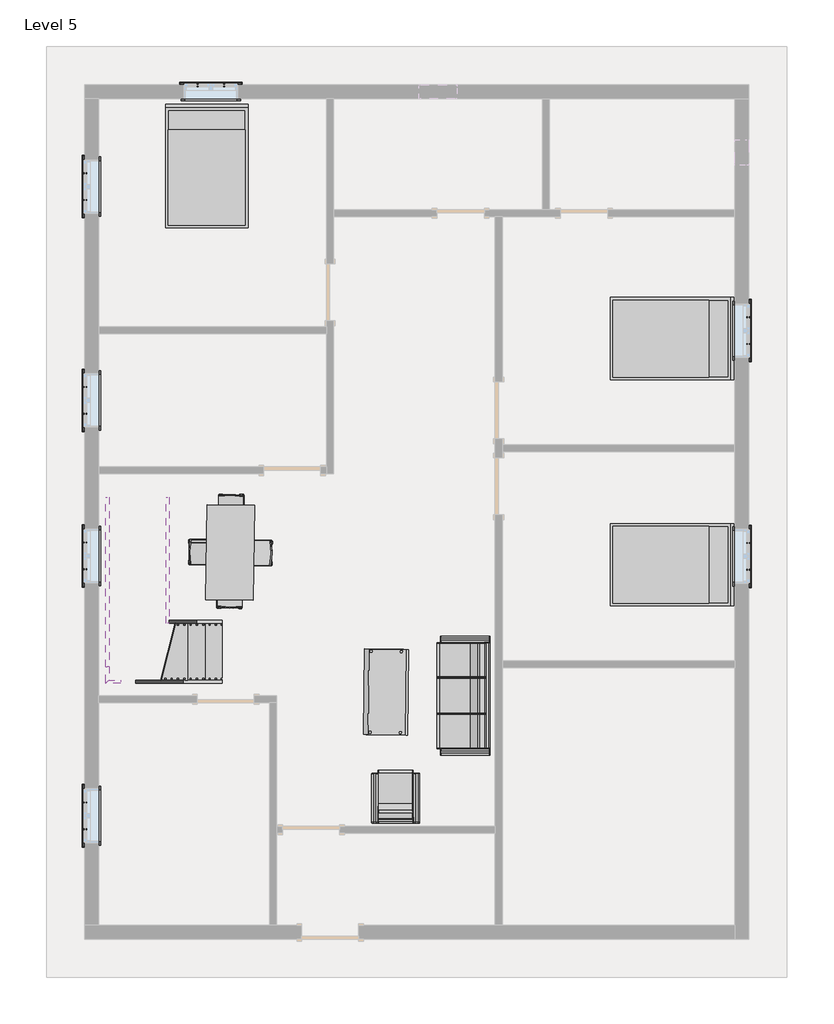
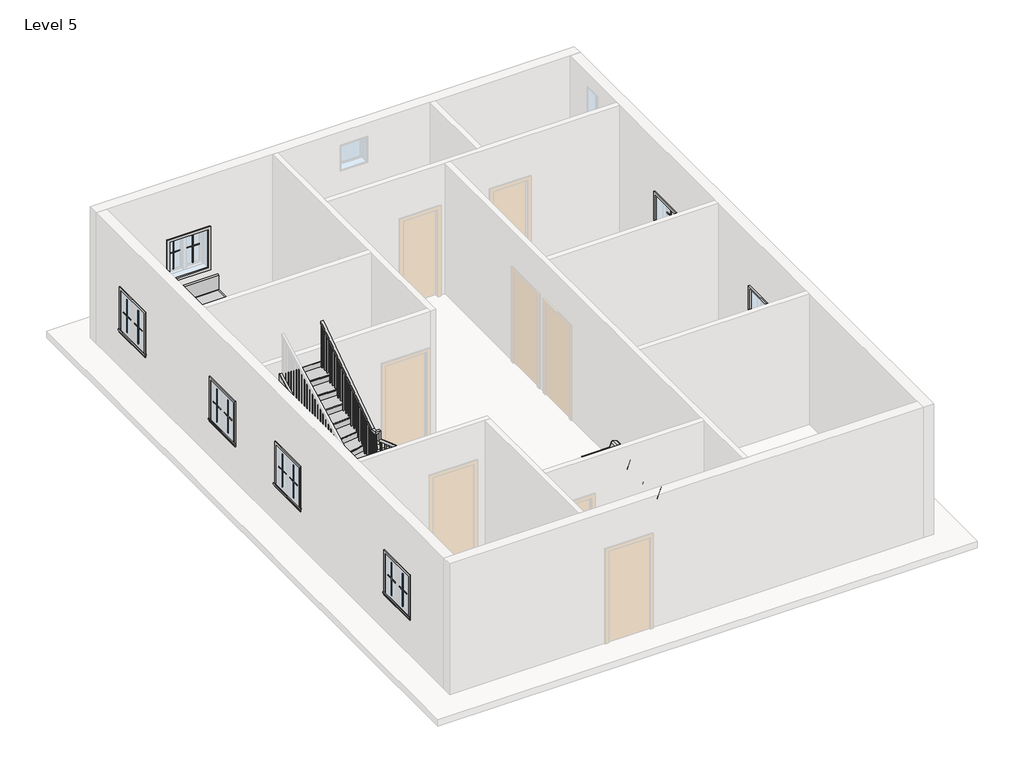
# One storey, part 2 of 2: 29 proxies, 6 furniture elements, 6 members, 1 railing, 1 stair flight.
"""IFC4 building model written with IfcOpenShell, lengths in millimetres."""

from ifc_helpers import new_model, si_unit, frame, origin, place, context, project, spatial, polyline, outline, extrude, faceted_brep, transform, mapped, element, save
from components import modern_coffee_table_17989_modern_coffee_table_17989_d3a860c8, muntin_pattern_2x2_muntin_pattern_2x2_b3fe6957, muntin_pattern_2x2_muntin_pattern_2x2_3e0ecaf2, trim_window_exterior_flat_with_sill_41619996, trim_window_interior_flat_picture_frame_51c85655, furniture_2fc85b74, furniture_29a9adb8, furniture_57072a26, furniture_f28dd14e, furniture_402a1f5e, bed_17739_bed_17739_15c61121, dining_table_w_chairs_11374_0cdfc61b, stair_flight_14253777

model = new_model("IFC4")

# Units and contexts
model_context = context("Model", 3, world=origin())
ifc_project = project(units=[si_unit("LENGTHUNIT", "METRE", prefix="MILLI")], contexts=[model_context])

# Site, building, storey
site = spatial("IfcSite", under=ifc_project)
building = spatial("IfcBuilding", under=site)
storey = spatial("IfcBuildingStorey", under=building, Name="Level 5", Elevation=9601.2)

# Proxies
placement = place(None, origin())
modern_coffee_table_17989_modern_coffee_table_17989_shape = modern_coffee_table_17989_modern_coffee_table_17989_d3a860c8(model_context)
element("IfcBuildingElementProxy", 1, Name="Modern_Coffee_Table_17989 : Modern_Coffee_Table_17989", ObjectType="Modern_Coffee_Table_17989 : Modern_Coffee_Table_17989", at=placement, inside=storey, context=model_context, shape_type="MappedRepresentation", body=[
    mapped(modern_coffee_table_17989_modern_coffee_table_17989_shape, transform((-2106.8718825, -2116.758017, 9601.2), x_axis=(0.012591066442684793, 0.9999207293810025, 0.0), y_axis=(-0.9999207293810025, 0.012591066442684793, 0.0), z_axis=(0.0, 0.0, 1.0))),
])
muntin_pattern_2x2_muntin_pattern_2x2_shape = muntin_pattern_2x2_muntin_pattern_2x2_b3fe6957(model_context)
element("IfcBuildingElementProxy", 2, Name="Muntin Pattern_2x2 : Muntin Pattern_2x2", ObjectType="Muntin Pattern_2x2 : Muntin Pattern_2x2", at=placement, inside=storey, context=model_context, shape_type="MappedRepresentation", body=[
    mapped(muntin_pattern_2x2_muntin_pattern_2x2_shape, transform((-4775.9474931, 7386.6685985, 10585.45), x_axis=(1.0, 0.0, 0.0), y_axis=(0.0, 1.0, 0.0), z_axis=(0.0, 0.0, 1.0))),
])
element("IfcBuildingElementProxy", 3, Name="Muntin Pattern_2x2 : Muntin Pattern_2x2", ObjectType="Muntin Pattern_2x2 : Muntin Pattern_2x2", at=placement, inside=storey, context=model_context, shape_type="MappedRepresentation", body=[
    mapped(muntin_pattern_2x2_muntin_pattern_2x2_shape, transform((4068.0150069, 3660.8060985, 10585.45), x_axis=(0.0, -1.0, 0.0), y_axis=(1.0, 0.0, 0.0), z_axis=(0.0, 0.0, 1.0))),
])
element("IfcBuildingElementProxy", 4, Name="Muntin Pattern_2x2 : Muntin Pattern_2x2", ObjectType="Muntin Pattern_2x2 : Muntin Pattern_2x2", at=placement, inside=storey, context=model_context, shape_type="MappedRepresentation", body=[
    mapped(muntin_pattern_2x2_muntin_pattern_2x2_shape, transform((4068.0150069, 40.9802908, 10585.45), x_axis=(0.0, -1.0, 0.0), y_axis=(1.0, 0.0, 0.0), z_axis=(0.0, 0.0, 1.0))),
])
element("IfcBuildingElementProxy", 5, Name="Muntin Pattern_2x2 : Muntin Pattern_2x2", ObjectType="Muntin Pattern_2x2 : Muntin Pattern_2x2", at=placement, inside=storey, context=model_context, shape_type="MappedRepresentation", body=[
    mapped(muntin_pattern_2x2_muntin_pattern_2x2_shape, transform((-6580.9349931, 2114.5810985, 10585.45), x_axis=(0.0, 1.0, 0.0), y_axis=(-1.0, 0.0, 0.0), z_axis=(0.0, 0.0, 1.0))),
])
element("IfcBuildingElementProxy", 6, Name="Muntin Pattern_2x2 : Muntin Pattern_2x2", ObjectType="Muntin Pattern_2x2 : Muntin Pattern_2x2", at=placement, inside=storey, context=model_context, shape_type="MappedRepresentation", body=[
    mapped(muntin_pattern_2x2_muntin_pattern_2x2_shape, transform((-6580.9349931, 5543.5810985, 10585.45), x_axis=(0.0, 1.0, 0.0), y_axis=(-1.0, 0.0, 0.0), z_axis=(0.0, 0.0, 1.0))),
])
element("IfcBuildingElementProxy", 7, Name="Muntin Pattern_2x2 : Muntin Pattern_2x2", ObjectType="Muntin Pattern_2x2 : Muntin Pattern_2x2", at=placement, inside=storey, context=model_context, shape_type="MappedRepresentation", body=[
    mapped(muntin_pattern_2x2_muntin_pattern_2x2_shape, transform((-6580.9349931, -4549.7439015, 10585.45), x_axis=(0.0, 1.0, 0.0), y_axis=(-1.0, 0.0, 0.0), z_axis=(0.0, 0.0, 1.0))),
])
element("IfcBuildingElementProxy", 8, Name="Muntin Pattern_2x2 : Muntin Pattern_2x2", ObjectType="Muntin Pattern_2x2 : Muntin Pattern_2x2", at=placement, inside=storey, context=model_context, shape_type="MappedRepresentation", body=[
    mapped(muntin_pattern_2x2_muntin_pattern_2x2_shape, transform((-6580.9349931, -380.9689015, 10585.45), x_axis=(0.0, 1.0, 0.0), y_axis=(-1.0, 0.0, 0.0), z_axis=(0.0, 0.0, 1.0))),
])
muntin_pattern_2x2_muntin_pattern_2x2_2_shape = muntin_pattern_2x2_muntin_pattern_2x2_3e0ecaf2(model_context)
element("IfcBuildingElementProxy", 9, Name="Muntin Pattern_2x2 : Muntin Pattern_2x2", ObjectType="Muntin Pattern_2x2 : Muntin Pattern_2x2", at=placement, inside=storey, context=model_context, shape_type="MappedRepresentation", body=[
    mapped(muntin_pattern_2x2_muntin_pattern_2x2_2_shape, transform((-4347.3224931, 7386.6685985, 10585.45), x_axis=(-1.0, 0.0, 0.0), y_axis=(0.0, -1.0, 0.0), z_axis=(0.0, 0.0, 1.0))),
])
element("IfcBuildingElementProxy", 10, Name="Muntin Pattern_2x2 : Muntin Pattern_2x2", ObjectType="Muntin Pattern_2x2 : Muntin Pattern_2x2", at=placement, inside=storey, context=model_context, shape_type="MappedRepresentation", body=[
    mapped(muntin_pattern_2x2_muntin_pattern_2x2_2_shape, transform((4068.0150069, 3232.1810985, 10585.45), x_axis=(0.0, 1.0, 0.0), y_axis=(-1.0, 0.0, 0.0), z_axis=(0.0, 0.0, 1.0))),
])
element("IfcBuildingElementProxy", 11, Name="Muntin Pattern_2x2 : Muntin Pattern_2x2", ObjectType="Muntin Pattern_2x2 : Muntin Pattern_2x2", at=placement, inside=storey, context=model_context, shape_type="MappedRepresentation", body=[
    mapped(muntin_pattern_2x2_muntin_pattern_2x2_2_shape, transform((4068.0150069, -387.6447092, 10585.45), x_axis=(0.0, 1.0, 0.0), y_axis=(-1.0, 0.0, 0.0), z_axis=(0.0, 0.0, 1.0))),
])
element("IfcBuildingElementProxy", 12, Name="Muntin Pattern_2x2 : Muntin Pattern_2x2", ObjectType="Muntin Pattern_2x2 : Muntin Pattern_2x2", at=placement, inside=storey, context=model_context, shape_type="MappedRepresentation", body=[
    mapped(muntin_pattern_2x2_muntin_pattern_2x2_2_shape, transform((-6580.9349931, 2543.2060985, 10585.45), x_axis=(0.0, -1.0, 0.0), y_axis=(1.0, 0.0, 0.0), z_axis=(0.0, 0.0, 1.0))),
])
element("IfcBuildingElementProxy", 13, Name="Muntin Pattern_2x2 : Muntin Pattern_2x2", ObjectType="Muntin Pattern_2x2 : Muntin Pattern_2x2", at=placement, inside=storey, context=model_context, shape_type="MappedRepresentation", body=[
    mapped(muntin_pattern_2x2_muntin_pattern_2x2_2_shape, transform((-6580.9349931, 5972.2060985, 10585.45), x_axis=(0.0, -1.0, 0.0), y_axis=(1.0, 0.0, 0.0), z_axis=(0.0, 0.0, 1.0))),
])
element("IfcBuildingElementProxy", 14, Name="Muntin Pattern_2x2 : Muntin Pattern_2x2", ObjectType="Muntin Pattern_2x2 : Muntin Pattern_2x2", at=placement, inside=storey, context=model_context, shape_type="MappedRepresentation", body=[
    mapped(muntin_pattern_2x2_muntin_pattern_2x2_2_shape, transform((-6580.9349931, -4121.1189015, 10585.45), x_axis=(0.0, -1.0, 0.0), y_axis=(1.0, 0.0, 0.0), z_axis=(0.0, 0.0, 1.0))),
])
element("IfcBuildingElementProxy", 15, Name="Muntin Pattern_2x2 : Muntin Pattern_2x2", ObjectType="Muntin Pattern_2x2 : Muntin Pattern_2x2", at=placement, inside=storey, context=model_context, shape_type="MappedRepresentation", body=[
    mapped(muntin_pattern_2x2_muntin_pattern_2x2_2_shape, transform((-6580.9349931, 47.6560985, 10585.45), x_axis=(0.0, -1.0, 0.0), y_axis=(1.0, 0.0, 0.0), z_axis=(0.0, 0.0, 1.0))),
])
trim_window_exterior_flat_with_sill_shape = trim_window_exterior_flat_with_sill_41619996(model_context)
element("IfcBuildingElementProxy", 16, Name="Trim-Window-Exterior-Flat : with Sill", ObjectType="Trim-Window-Exterior-Flat : with Sill", at=placement, inside=storey, context=model_context, shape_type="MappedRepresentation", body=[
    mapped(trim_window_exterior_flat_with_sill_shape, transform((-4561.6349931, 7396.1935985, 11430.0), x_axis=(-1.0, 0.0, 0.0), y_axis=(0.0, 0.0, 1.0), z_axis=(0.0, 1.0, 0.0))),
])
element("IfcBuildingElementProxy", 17, Name="Trim-Window-Exterior-Flat : with Sill", ObjectType="Trim-Window-Exterior-Flat : with Sill", at=placement, inside=storey, context=model_context, shape_type="MappedRepresentation", body=[
    mapped(trim_window_exterior_flat_with_sill_shape, transform((4077.5400069, 3446.4935985, 11430.0), x_axis=(0.0, 1.0, 0.0), y_axis=(0.0, 0.0, 1.0), z_axis=(1.0, 0.0, 0.0))),
])
element("IfcBuildingElementProxy", 18, Name="Trim-Window-Exterior-Flat : with Sill", ObjectType="Trim-Window-Exterior-Flat : with Sill", at=placement, inside=storey, context=model_context, shape_type="MappedRepresentation", body=[
    mapped(trim_window_exterior_flat_with_sill_shape, transform((4077.5400069, -173.3322092, 11430.0), x_axis=(0.0, 1.0, 0.0), y_axis=(0.0, 0.0, 1.0), z_axis=(1.0, 0.0, 0.0))),
])
element("IfcBuildingElementProxy", 19, Name="Trim-Window-Exterior-Flat : with Sill", ObjectType="Trim-Window-Exterior-Flat : with Sill", at=placement, inside=storey, context=model_context, shape_type="MappedRepresentation", body=[
    mapped(trim_window_exterior_flat_with_sill_shape, transform((-6590.4599931, 2328.8935985, 11430.0), x_axis=(0.0, -1.0, 0.0), y_axis=(0.0, 0.0, 1.0), z_axis=(-1.0, 0.0, 0.0))),
])
element("IfcBuildingElementProxy", 20, Name="Trim-Window-Exterior-Flat : with Sill", ObjectType="Trim-Window-Exterior-Flat : with Sill", at=placement, inside=storey, context=model_context, shape_type="MappedRepresentation", body=[
    mapped(trim_window_exterior_flat_with_sill_shape, transform((-6590.4599931, 5757.8935985, 11430.0), x_axis=(0.0, -1.0, 0.0), y_axis=(0.0, 0.0, 1.0), z_axis=(-1.0, 0.0, 0.0))),
])
element("IfcBuildingElementProxy", 21, Name="Trim-Window-Exterior-Flat : with Sill", ObjectType="Trim-Window-Exterior-Flat : with Sill", at=placement, inside=storey, context=model_context, shape_type="MappedRepresentation", body=[
    mapped(trim_window_exterior_flat_with_sill_shape, transform((-6590.4599931, -4335.4314015, 11430.0), x_axis=(0.0, -1.0, 0.0), y_axis=(0.0, 0.0, 1.0), z_axis=(-1.0, 0.0, 0.0))),
])
element("IfcBuildingElementProxy", 22, Name="Trim-Window-Exterior-Flat : with Sill", ObjectType="Trim-Window-Exterior-Flat : with Sill", at=placement, inside=storey, context=model_context, shape_type="MappedRepresentation", body=[
    mapped(trim_window_exterior_flat_with_sill_shape, transform((-6590.4599931, -166.6564015, 11430.0), x_axis=(0.0, -1.0, 0.0), y_axis=(0.0, 0.0, 1.0), z_axis=(-1.0, 0.0, 0.0))),
])
trim_window_interior_flat_picture_frame_shape = trim_window_interior_flat_picture_frame_51c85655(model_context)
element("IfcBuildingElementProxy", 23, Name="Trim-Window-Interior-Flat : Picture Frame", ObjectType="Trim-Window-Interior-Flat : Picture Frame", at=placement, inside=storey, context=model_context, shape_type="MappedRepresentation", body=[
    mapped(trim_window_interior_flat_picture_frame_shape, transform((-4561.6349931, 7167.5935985, 11430.0), x_axis=(1.0, 0.0, 0.0), y_axis=(0.0, 0.0, 1.0), z_axis=(0.0, -1.0, 0.0))),
])
element("IfcBuildingElementProxy", 24, Name="Trim-Window-Interior-Flat : Picture Frame", ObjectType="Trim-Window-Interior-Flat : Picture Frame", at=placement, inside=storey, context=model_context, shape_type="MappedRepresentation", body=[
    mapped(trim_window_interior_flat_picture_frame_shape, transform((3848.9400069, 3446.4935985, 11430.0), x_axis=(0.0, -1.0, 0.0), y_axis=(0.0, 0.0, 1.0), z_axis=(-1.0, 0.0, 0.0))),
])
element("IfcBuildingElementProxy", 25, Name="Trim-Window-Interior-Flat : Picture Frame", ObjectType="Trim-Window-Interior-Flat : Picture Frame", at=placement, inside=storey, context=model_context, shape_type="MappedRepresentation", body=[
    mapped(trim_window_interior_flat_picture_frame_shape, transform((3848.9400069, -173.3322092, 11430.0), x_axis=(0.0, -1.0, 0.0), y_axis=(0.0, 0.0, 1.0), z_axis=(-1.0, 0.0, 0.0))),
])
element("IfcBuildingElementProxy", 26, Name="Trim-Window-Interior-Flat : Picture Frame", ObjectType="Trim-Window-Interior-Flat : Picture Frame", at=placement, inside=storey, context=model_context, shape_type="MappedRepresentation", body=[
    mapped(trim_window_interior_flat_picture_frame_shape, transform((-6361.8599931, 2328.8935985, 11430.0), x_axis=(0.0, 1.0, 0.0), y_axis=(0.0, 0.0, 1.0), z_axis=(1.0, 0.0, 0.0))),
])
element("IfcBuildingElementProxy", 27, Name="Trim-Window-Interior-Flat : Picture Frame", ObjectType="Trim-Window-Interior-Flat : Picture Frame", at=placement, inside=storey, context=model_context, shape_type="MappedRepresentation", body=[
    mapped(trim_window_interior_flat_picture_frame_shape, transform((-6361.8599931, 5757.8935985, 11430.0), x_axis=(0.0, 1.0, 0.0), y_axis=(0.0, 0.0, 1.0), z_axis=(1.0, 0.0, 0.0))),
])
element("IfcBuildingElementProxy", 28, Name="Trim-Window-Interior-Flat : Picture Frame", ObjectType="Trim-Window-Interior-Flat : Picture Frame", at=placement, inside=storey, context=model_context, shape_type="MappedRepresentation", body=[
    mapped(trim_window_interior_flat_picture_frame_shape, transform((-6361.8599931, -4335.4314015, 11430.0), x_axis=(0.0, 1.0, 0.0), y_axis=(0.0, 0.0, 1.0), z_axis=(1.0, 0.0, 0.0))),
])
element("IfcBuildingElementProxy", 29, Name="Trim-Window-Interior-Flat : Picture Frame", ObjectType="Trim-Window-Interior-Flat : Picture Frame", at=placement, inside=storey, context=model_context, shape_type="MappedRepresentation", body=[
    mapped(trim_window_interior_flat_picture_frame_shape, transform((-6361.8599931, -166.6564015, 11430.0), x_axis=(0.0, 1.0, 0.0), y_axis=(0.0, 0.0, 1.0), z_axis=(1.0, 0.0, 0.0))),
])

# Furniture
furniture_shape = furniture_2fc85b74(model_context)
furniture_2_shape = furniture_29a9adb8(model_context)
furniture_3_shape = furniture_57072a26(model_context)
element("IfcFurniture", 30, at=placement, inside=storey, context=model_context, shape_type="MappedRepresentation", body=[
    mapped(furniture_shape, transform((-877.7263413, -2408.2064015, 9601.2), x_axis=(0.0, -1.0, 0.0), y_axis=(1.0, 0.0, 0.0), z_axis=(0.0, 0.0, 1.0))),
    mapped(furniture_2_shape, transform((-877.7263413, -2408.2064015, 9601.2), x_axis=(0.0, -1.0, 0.0), y_axis=(1.0, 0.0, 0.0), z_axis=(0.0, 0.0, 1.0))),
    mapped(furniture_3_shape, transform((-877.7263413, -2408.2064015, 9601.2), x_axis=(0.0, -1.0, 0.0), y_axis=(1.0, 0.0, 0.0), z_axis=(0.0, 0.0, 1.0))),
])
furniture_4_shape = furniture_f28dd14e(model_context)
furniture_5_shape = furniture_402a1f5e(model_context)
element("IfcFurniture", 31, at=placement, inside=storey, context=model_context, shape_type="MappedRepresentation", body=[
    mapped(furniture_4_shape, transform((-1595.4975416, -3653.2527501, 9601.2), x_axis=(-1.0, 0.0, 0.0), y_axis=(0.0, -1.0, 0.0), z_axis=(0.0, 0.0, 1.0))),
    mapped(furniture_5_shape, transform((-1595.4975416, -3653.2527501, 9601.2), x_axis=(-1.0, 0.0, 0.0), y_axis=(0.0, -1.0, 0.0), z_axis=(0.0, 0.0, 1.0))),
])
bed_17739_bed_17739_shape = bed_17739_bed_17739_15c61121(model_context)
element("IfcFurniture", 32, ObjectType="Bed_17739 : Bed_17739", at=placement, inside=storey, context=model_context, shape_type="MappedRepresentation", body=[
    mapped(bed_17739_bed_17739_shape, transform((-4628.3099931, 6062.6935985, 9601.2), x_axis=(1.0, 0.0, 0.0), y_axis=(0.0, 1.0, 0.0), z_axis=(0.0, 0.0, 1.0))),
])
element("IfcFurniture", 33, ObjectType="Bed_17739 : Bed_17739", at=placement, inside=storey, context=model_context, shape_type="MappedRepresentation", body=[
    mapped(bed_17739_bed_17739_shape, transform((2820.2400069, 3319.4935985, 9601.2), x_axis=(0.0, -1.0, 0.0), y_axis=(1.0, 0.0, 0.0), z_axis=(0.0, 0.0, 1.0))),
])
element("IfcFurniture", 34, ObjectType="Bed_17739 : Bed_17739", at=placement, inside=storey, context=model_context, shape_type="MappedRepresentation", body=[
    mapped(bed_17739_bed_17739_shape, transform((2820.2400069, -307.008017, 9601.2), x_axis=(0.0, -1.0, 0.0), y_axis=(1.0, 0.0, 0.0), z_axis=(0.0, 0.0, 1.0))),
])
dining_table_w_chairs_11374_shape = dining_table_w_chairs_11374_0cdfc61b(model_context)
element("IfcFurniture", 35, ObjectType="Dining_Table_w_Chairs_11374", at=placement, inside=storey, context=model_context, shape_type="MappedRepresentation", body=[
    mapped(dining_table_w_chairs_11374_shape, transform((-4154.6586335, -131.9172641, 9601.2), x_axis=(0.015873758475140665, 0.9998740039584353, 0.0), y_axis=(-0.9998740039584353, 0.015873758475140665, 0.0), z_axis=(0.0, 0.0, 1.0))),
])

# Members
element("IfcMember", 36, ObjectType="Stringer - 2\" Width", at=placement, inside=storey, context=model_context, shape_type="SweptSolid", body=[
    extrude(outline(polyline([(10191.2562463, -4378.4230036), (10524.0849999, -4378.4230036), (11239.2971411, -6009.0851964), (10906.4683876, -6009.0851964), (10191.2562463, -4378.4230036)])), frame((0.0, -2211.3564015, 0.0), z_axis=(0.0, 1.0, 0.0), x_axis=(0.0, 0.0, 1.0)), (0.0, 0.0, 1.0), 50.8),
])
element("IfcMember", 37, ObjectType="Stringer - 2\" Width", at=placement, inside=storey, context=model_context, shape_type="SweptSolid", body=[
    extrude(outline(polyline([(-6009.0851964, -2160.5564015), (-6009.0851964, -2211.3564015), (-6247.5599931, -2211.3564015), (-6196.7599931, -2160.5564015), (-6009.0851964, -2160.5564015)])), frame((0.0, 0.0, 10906.4683876), z_axis=(0.0, 0.0, 1.0), x_axis=(1.0, 0.0, 0.0)), (0.0, 0.0, 1.0), 332.8287535),
])
element("IfcMember", 38, ObjectType="Stringer - 2\" Width", at=placement, inside=storey, context=model_context, shape_type="SweptSolid", body=[
    extrude(outline(polyline([(-6196.7599931, -2160.5564015), (-6247.5599931, -2211.3564015), (-6247.5599931, -1942.4030584), (-6196.7599931, -1942.4030584), (-6196.7599931, -2160.5564015)])), frame((0.0, 0.0, 10906.4683876), z_axis=(0.0, 0.0, 1.0), x_axis=(1.0, 0.0, 0.0)), (0.0, 0.0, 1.0), 332.8287535),
])
element("IfcMember", 39, ObjectType="Stringer - 2\" Width", at=placement, inside=storey, context=model_context, shape_type="SweptSolid", body=[
    extrude(outline(polyline([(-1942.4030584, 10906.4683876), (-1942.4030584, 11239.2971411), (775.380588, 12654.8189504), (775.380588, 12321.9901969), (-1942.4030584, 10906.4683876)])), frame((-6247.5599931, 0.0, 0.0), z_axis=(1.0, 0.0, 0.0), x_axis=(0.0, 1.0, 0.0)), (0.0, 0.0, 1.0), 50.8),
])
element("IfcMember", 40, ObjectType="Stringer - 2\" Width", at=placement, inside=storey, context=model_context, shape_type="SweptSolid", body=[
    extrude(outline(polyline([(10036.6922729, -4378.4230036), (10443.834734, -4378.4230036), (11199.3690344, -5231.5599931), (10792.2265733, -5231.5599931), (10036.6922729, -4378.4230036)])), frame((0.0, -1246.1564015, 0.0), z_axis=(0.0, 1.0, 0.0), x_axis=(0.0, 0.0, 1.0)), (0.0, 0.0, 1.0), 50.8),
])
element("IfcMember", 41, ObjectType="Stringer - 2\" Width", at=placement, inside=storey, context=model_context, shape_type="SweptSolid", body=[
    extrude(outline(polyline([(-1246.1564015, 10938.9212805), (-1246.1564015, 11311.1296678), (775.380588, 12727.9693854), (775.380588, 12355.7609981), (-1246.1564015, 10938.9212805)])), frame((-5282.3599931, 0.0, 0.0), z_axis=(1.0, 0.0, 0.0), x_axis=(0.0, 1.0, 0.0)), (0.0, 0.0, 1.0), 50.8),
])

# Railing
element("IfcRailing", 42, ObjectType="Handrail - Rectangular", at=placement, inside=storey, context=model_context, shape_type="SolidModel", body=[
    faceted_brep([(-4378.4230036, -1296.9564015, 11362.2666667), (-4378.4230036, -1296.9564015, 11297.3997378), (-4378.4230036, -1246.1564015, 11297.3997378), (-4378.4230036, -1246.1564015, 11362.2666667), (-5206.1599931, -1296.9564015, 12019.5201542), (-5256.9599931, -1296.9564015, 11994.990286), (-5256.9599931, -1246.1564015, 11994.990286), (-5206.1599931, -1246.1564015, 12019.5201542), (-5206.1599931, -1296.9564015, 12226.3172738), (-5256.9599931, -1296.9564015, 12175.5172738), (-5256.9599931, -1246.1564015, 12175.5172738), (-5206.1599931, -1246.1564015, 12226.3172738), (-5333.1599931, -1296.9564015, 12226.3172738), (-5333.1599931, -1296.9564015, 12175.5172738), (-5282.3599931, -1246.1564015, 12175.5172738), (-5282.3599931, -1246.1564015, 12226.3172738), (-5333.1599931, -1169.9564015, 12226.3172738), (-5333.1599931, -1154.1797661, 12175.5172738), (-5282.3599931, -1154.1797661, 12175.5172738), (-5282.3599931, -1169.9564015, 12226.3172738), (-5333.1599931, 775.380588, 13563.6), (-5282.3599931, 775.380588, 13563.6), (-5282.3599931, 775.380588, 13501.9546698), (-5333.1599931, 775.380588, 13501.9546698)], [[[0, 1, 2, 3]], [[1, 0, 4, 5]], [[2, 1, 5, 6]], [[3, 2, 6, 7]], [[0, 3, 7, 4]], [[5, 4, 8, 9]], [[6, 5, 9, 10]], [[7, 6, 10, 11]], [[4, 7, 11, 8]], [[9, 8, 12, 13]], [[10, 9, 13, 14]], [[11, 10, 14, 15]], [[8, 11, 15, 12]], [[13, 12, 16, 17]], [[14, 13, 17, 18]], [[15, 14, 18, 19]], [[12, 15, 19, 16]], [[20, 21, 22, 23]], [[17, 16, 20, 23]], [[18, 17, 23, 22]], [[19, 18, 22, 21]], [[16, 19, 21, 20]]]),
    extrude(outline(polyline([(750.9185985, 13485.1387679), (769.9685985, 13498.2343066), (769.9685985, 12479.8666667), (750.9185985, 12479.8666667), (750.9185985, 13485.1387679)])), frame((-5317.2849931, 0.0, 0.0), z_axis=(1.0, 0.0, 0.0), x_axis=(0.0, 1.0, 0.0)), (0.0, 0.0, 1.0), 19.05),
    extrude(outline(polyline([(649.3185985, 13415.2958945), (668.3685985, 13428.3914333), (668.3685985, 12479.8666667), (649.3185985, 12479.8666667), (649.3185985, 13415.2958945)])), frame((-5317.2849931, 0.0, 0.0), z_axis=(1.0, 0.0, 0.0), x_axis=(0.0, 1.0, 0.0)), (0.0, 0.0, 1.0), 19.05),
    extrude(outline(polyline([(547.7185985, 13345.4530212), (566.7685985, 13358.5485599), (566.7685985, 12479.8666667), (547.7185985, 12479.8666667), (547.7185985, 13345.4530212)])), frame((-5317.2849931, 0.0, 0.0), z_axis=(1.0, 0.0, 0.0), x_axis=(0.0, 1.0, 0.0)), (0.0, 0.0, 1.0), 19.05),
    extrude(outline(polyline([(446.1185985, 13275.6101478), (465.1685985, 13288.7056866), (465.1685985, 12310.5333333), (446.1185985, 12310.5333333), (446.1185985, 13275.6101478)])), frame((-5317.2849931, 0.0, 0.0), z_axis=(1.0, 0.0, 0.0), x_axis=(0.0, 1.0, 0.0)), (0.0, 0.0, 1.0), 19.05),
    extrude(outline(polyline([(344.5185985, 13205.7672745), (363.5685985, 13218.8628132), (363.5685985, 12310.5333333), (344.5185985, 12310.5333333), (344.5185985, 13205.7672745)])), frame((-5317.2849931, 0.0, 0.0), z_axis=(1.0, 0.0, 0.0), x_axis=(0.0, 1.0, 0.0)), (0.0, 0.0, 1.0), 19.05),
    extrude(outline(polyline([(242.9185985, 13135.9244011), (261.9685985, 13149.0199399), (261.9685985, 12310.5333333), (242.9185985, 12310.5333333), (242.9185985, 13135.9244011)])), frame((-5317.2849931, 0.0, 0.0), z_axis=(1.0, 0.0, 0.0), x_axis=(0.0, 1.0, 0.0)), (0.0, 0.0, 1.0), 19.05),
    extrude(outline(polyline([(141.3185985, 13066.0815278), (160.3685985, 13079.1770665), (160.3685985, 12141.2), (141.3185985, 12141.2), (141.3185985, 13066.0815278)])), frame((-5317.2849931, 0.0, 0.0), z_axis=(1.0, 0.0, 0.0), x_axis=(0.0, 1.0, 0.0)), (0.0, 0.0, 1.0), 19.05),
    extrude(outline(polyline([(39.7185985, 12996.2386544), (58.7685985, 13009.3341932), (58.7685985, 12141.2), (39.7185985, 12141.2), (39.7185985, 12996.2386544)])), frame((-5317.2849931, 0.0, 0.0), z_axis=(1.0, 0.0, 0.0), x_axis=(0.0, 1.0, 0.0)), (0.0, 0.0, 1.0), 19.05),
    extrude(outline(polyline([(-61.8814015, 12926.3957811), (-42.8314015, 12939.4913198), (-42.8314015, 11971.8666667), (-61.8814015, 11971.8666667), (-61.8814015, 12926.3957811)])), frame((-5317.2849931, 0.0, 0.0), z_axis=(1.0, 0.0, 0.0), x_axis=(0.0, 1.0, 0.0)), (0.0, 0.0, 1.0), 19.05),
    extrude(outline(polyline([(-163.4814015, 12856.5529077), (-144.4314015, 12869.6484465), (-144.4314015, 11971.8666667), (-163.4814015, 11971.8666667), (-163.4814015, 12856.5529077)])), frame((-5317.2849931, 0.0, 0.0), z_axis=(1.0, 0.0, 0.0), x_axis=(0.0, 1.0, 0.0)), (0.0, 0.0, 1.0), 19.05),
    extrude(outline(polyline([(-265.0814015, 12786.7100344), (-246.0314015, 12799.8055731), (-246.0314015, 11971.8666667), (-265.0814015, 11971.8666667), (-265.0814015, 12786.7100344)])), frame((-5317.2849931, 0.0, 0.0), z_axis=(1.0, 0.0, 0.0), x_axis=(0.0, 1.0, 0.0)), (0.0, 0.0, 1.0), 19.05),
    extrude(outline(polyline([(-366.6814015, 12716.867161), (-347.6314015, 12729.9626998), (-347.6314015, 11802.5333333), (-366.6814015, 11802.5333333), (-366.6814015, 12716.867161)])), frame((-5317.2849931, 0.0, 0.0), z_axis=(1.0, 0.0, 0.0), x_axis=(0.0, 1.0, 0.0)), (0.0, 0.0, 1.0), 19.05),
    extrude(outline(polyline([(-468.2814015, 12647.0242877), (-449.2314015, 12660.1198264), (-449.2314015, 11802.5333333), (-468.2814015, 11802.5333333), (-468.2814015, 12647.0242877)])), frame((-5317.2849931, 0.0, 0.0), z_axis=(1.0, 0.0, 0.0), x_axis=(0.0, 1.0, 0.0)), (0.0, 0.0, 1.0), 19.05),
    extrude(outline(polyline([(-569.8814015, 12577.1814143), (-550.8314015, 12590.2769531), (-550.8314015, 11802.5333333), (-569.8814015, 11802.5333333), (-569.8814015, 12577.1814143)])), frame((-5317.2849931, 0.0, 0.0), z_axis=(1.0, 0.0, 0.0), x_axis=(0.0, 1.0, 0.0)), (0.0, 0.0, 1.0), 19.05),
    extrude(outline(polyline([(-671.4814015, 12507.338541), (-652.4314015, 12520.4340797), (-652.4314015, 11633.2), (-671.4814015, 11633.2), (-671.4814015, 12507.338541)])), frame((-5317.2849931, 0.0, 0.0), z_axis=(1.0, 0.0, 0.0), x_axis=(0.0, 1.0, 0.0)), (0.0, 0.0, 1.0), 19.05),
    extrude(outline(polyline([(-773.0814015, 12437.4956676), (-754.0314015, 12450.5912064), (-754.0314015, 11633.2), (-773.0814015, 11633.2), (-773.0814015, 12437.4956676)])), frame((-5317.2849931, 0.0, 0.0), z_axis=(1.0, 0.0, 0.0), x_axis=(0.0, 1.0, 0.0)), (0.0, 0.0, 1.0), 19.05),
    extrude(outline(polyline([(-874.6814015, 12367.6527943), (-855.6314015, 12380.748333), (-855.6314015, 11463.8666667), (-874.6814015, 11463.8666667), (-874.6814015, 12367.6527943)])), frame((-5317.2849931, 0.0, 0.0), z_axis=(1.0, 0.0, 0.0), x_axis=(0.0, 1.0, 0.0)), (0.0, 0.0, 1.0), 19.05),
    extrude(outline(polyline([(-976.2814015, 12297.8099209), (-957.2314015, 12310.9054597), (-957.2314015, 11463.8666667), (-976.2814015, 11463.8666667), (-976.2814015, 12297.8099209)])), frame((-5317.2849931, 0.0, 0.0), z_axis=(1.0, 0.0, 0.0), x_axis=(0.0, 1.0, 0.0)), (0.0, 0.0, 1.0), 19.05),
    extrude(outline(polyline([(-1077.8814015, 12227.9670476), (-1058.8314015, 12241.0625863), (-1058.8314015, 11294.5333333), (-1077.8814015, 11294.5333333), (-1077.8814015, 12227.9670476)])), frame((-5317.2849931, 0.0, 0.0), z_axis=(1.0, 0.0, 0.0), x_axis=(0.0, 1.0, 0.0)), (0.0, 0.0, 1.0), 19.05),
    extrude(outline(polyline([(-1179.4814015, 12158.1241742), (-1160.4314015, 12171.219713), (-1160.4314015, 11294.5333333), (-1179.4814015, 11294.5333333), (-1179.4814015, 12158.1241742)])), frame((-5317.2849931, 0.0, 0.0), z_axis=(1.0, 0.0, 0.0), x_axis=(0.0, 1.0, 0.0)), (0.0, 0.0, 1.0), 19.05),
    extrude(outline(polyline([(-5283.2980036, -1262.0314015), (-5283.2980036, -1281.0814015), (-5302.3480036, -1281.0814015), (-5302.3480036, -1262.0314015), (-5283.2980036, -1262.0314015)])), frame((0.0, 0.0, 11125.2), z_axis=(0.0, 0.0, 1.0), x_axis=(1.0, 0.0, 0.0)), (0.0, 0.0, 1.0), 1050.3172738),
    extrude(outline(polyline([(11935.2295097, -5181.6980036), (11950.3559074, -5200.7480036), (10955.8666667, -5200.7480036), (10955.8666667, -5181.6980036), (11935.2295097, -5181.6980036)])), frame((0.0, -1281.0814015, 0.0), z_axis=(0.0, 1.0, 0.0), x_axis=(0.0, 0.0, 1.0)), (0.0, 0.0, 1.0), 19.05),
    extrude(outline(polyline([(11854.5553883, -5080.0980036), (11869.6817861, -5099.1480036), (10786.5333333, -5099.1480036), (10786.5333333, -5080.0980036), (11854.5553883, -5080.0980036)])), frame((0.0, -1281.0814015, 0.0), z_axis=(0.0, 1.0, 0.0), x_axis=(0.0, 0.0, 1.0)), (0.0, 0.0, 1.0), 19.05),
    extrude(outline(polyline([(11773.881267, -4978.4980036), (11789.0076647, -4997.5480036), (10786.5333333, -4997.5480036), (10786.5333333, -4978.4980036), (11773.881267, -4978.4980036)])), frame((0.0, -1281.0814015, 0.0), z_axis=(0.0, 1.0, 0.0), x_axis=(0.0, 0.0, 1.0)), (0.0, 0.0, 1.0), 19.05),
    extrude(outline(polyline([(11693.2071456, -4876.8980036), (11708.3335434, -4895.9480036), (10617.2, -4895.9480036), (10617.2, -4876.8980036), (11693.2071456, -4876.8980036)])), frame((0.0, -1281.0814015, 0.0), z_axis=(0.0, 1.0, 0.0), x_axis=(0.0, 0.0, 1.0)), (0.0, 0.0, 1.0), 19.05),
    extrude(outline(polyline([(11612.5330243, -4775.2980036), (11627.659422, -4794.3480036), (10617.2, -4794.3480036), (10617.2, -4775.2980036), (11612.5330243, -4775.2980036)])), frame((0.0, -1281.0814015, 0.0), z_axis=(0.0, 1.0, 0.0), x_axis=(0.0, 0.0, 1.0)), (0.0, 0.0, 1.0), 19.05),
    extrude(outline(polyline([(11531.8589029, -4673.6980036), (11546.9853007, -4692.7480036), (10617.2, -4692.7480036), (10617.2, -4673.6980036), (11531.8589029, -4673.6980036)])), frame((0.0, -1281.0814015, 0.0), z_axis=(0.0, 1.0, 0.0), x_axis=(0.0, 0.0, 1.0)), (0.0, 0.0, 1.0), 19.05),
    extrude(outline(polyline([(11451.1847816, -4572.0980036), (11466.3111793, -4591.1480036), (10447.8666667, -4591.1480036), (10447.8666667, -4572.0980036), (11451.1847816, -4572.0980036)])), frame((0.0, -1281.0814015, 0.0), z_axis=(0.0, 1.0, 0.0), x_axis=(0.0, 0.0, 1.0)), (0.0, 0.0, 1.0), 19.05),
    extrude(outline(polyline([(11370.5106602, -4470.4980036), (11385.637058, -4489.5480036), (10447.8666667, -4489.5480036), (10447.8666667, -4470.4980036), (11370.5106602, -4470.4980036)])), frame((0.0, -1281.0814015, 0.0), z_axis=(0.0, 1.0, 0.0), x_axis=(0.0, 0.0, 1.0)), (0.0, 0.0, 1.0), 19.05),
    extrude(outline(polyline([(-5298.2349931, -1262.0314015), (-5298.2349931, -1281.0814015), (-5317.2849931, -1281.0814015), (-5317.2849931, -1262.0314015), (-5298.2349931, -1262.0314015)])), frame((0.0, 0.0, 11125.2), z_axis=(0.0, 0.0, 1.0), x_axis=(1.0, 0.0, 0.0)), (0.0, 0.0, 1.0), 1050.3172738),
    extrude(outline(polyline([(756.330588, 13488.859131), (775.380588, 13501.9546698), (775.380588, 12479.8666667), (756.330588, 12479.8666667), (756.330588, 13488.859131)])), frame((-5317.2849931, 0.0, 0.0), z_axis=(1.0, 0.0, 0.0), x_axis=(0.0, 1.0, 0.0)), (0.0, 0.0, 1.0), 19.05),
    extrude(outline(polyline([(11297.3997378, -4378.4230036), (11312.5261355, -4397.4730036), (10447.8666667, -4397.4730036), (10447.8666667, -4378.4230036), (11297.3997378, -4378.4230036)])), frame((0.0, -1281.0814015, 0.0), z_axis=(0.0, 1.0, 0.0), x_axis=(0.0, 0.0, 1.0)), (0.0, 0.0, 1.0), 19.05),
])

# Stair flight
stair_flight_shape = stair_flight_14253777(model_context)
element("IfcStairFlight", 43, ObjectType="2\" Tread 1\" Nosing 1/4\" Riser", at=placement, inside=storey, context=model_context, shape_type="MappedRepresentation", body=[
    mapped(stair_flight_shape, transform((0.0, 0.0, 0.0), x_axis=(1.0, 0.0, 0.0), y_axis=(0.0, 1.0, 0.0), z_axis=(0.0, 0.0, 1.0))),
])

save(model, "model.ifc")

# Revit data of these elements
# Type "Modern_Coffee_Table_17989 : Modern_Coffee_Table_17989"
#   Default Elevation = 0
# Type "Muntin Pattern_2x2 : Muntin Pattern_2x2"
#   Width [instance default] = 4' - 0"
#   Thickness = 0' - 0 1/2"
#   Height [instance default] = 4' - 0"
#   Distance = 0' - 0 3/4"
#   Interior Material [instance default] = none
#   Exterior Material [instance default] = none
#   Default Elevation = 0
# Type "Trim-Window-Exterior-Flat : with Sill"
#   Trim Width = 0' - 2 1/4"
#   Trim Thickness_Picture Frame = 0' - 1 1/4"
#   Trim Thickness_with Sill = 0' - 0 3/4"
#   Sill Thickness = 0' - 1 1/4"
#   Opening Width [instance default] = 2' - 0"
#   Opening Height [instance default] = 3' - 0"
#   Default Elevation = 4' - 0"
#   Sill = yes
#   Picture Frame = no
#   Trim Material [instance default] = none
# Type "Trim-Window-Interior-Flat : Picture Frame"
#   Trim Thickness_Picture Frame = 0' - 1 1/4"
#   Trim Width = 0' - 2 1/4"
#   Trim Thickness_with Sill = 0' - 0 3/4"
#   Sill Thickness = 0' - 1 1/4"
#   Opening Width [instance default] = 2' - 0"
#   Opening Height [instance default] = 3' - 0"
#   Default Elevation = 4' - 0"
#   Sill = no
#   Picture Frame = yes
#   Trim Material [instance default] = none
# Type
#   Width [instance] = 6' - 3.19685"
#   Default Elevation = 0
# Type
#   Width [instance] = 2' - 6.31496"
#   Default Elevation = 0
# Type "Bed_17739 : Bed_17739"
#   Default Elevation = 0
# Type "Dining_Table_w_Chairs_11374"
#   Default Elevation = 0
#   Assembly Code = ""
# Type "Handrail - Rectangular"
#   Assembly Code = "C2010400"
#   built-in parameter 1008612 = 0.0416667 (stored number, unit not read)
#   built-in parameter 1008611 = 0.0416667 (stored number, unit not read)
#   built-in parameter 1008609 = 0.333333 (stored number, unit not read)
#   built-in parameter 1008604 = 0.166667 (stored number, unit not read)
#   built-in parameter 1008603 = 0.166667 (stored number, unit not read)
#   Railing Height = 3' - 0"
#   built-in parameter 1008630 = 2
#   built-in parameter 1008610 = 2
#   built-in parameter 1008618 = Baluster - Square : 3/4"
# Element 1 (IfcBuildingElementProxy, "Modern_Coffee_Table_17989 : Modern_Coffee_Table_17989")
#   Phase Created = New Construction
#   Materials on its faces: "1 Wood", "1 Glass", "1 Metal"
# Elements 2, 3, 4, 5, 6, 7, 8, 9, 10, 11, 12, 13, 14, 15 (IfcBuildingElementProxy, "Muntin Pattern_2x2 : Muntin Pattern_2x2")
#   Width = 0' - 11 5/8"
#   Height = 2' - 6 1/2"
#   Interior Material = Wood - Stained
#   Exterior Material = Clad - White
#   Phase Created = New Construction
#   Materials on its faces: "Clad - White", "Wood - Stained"
# Elements 16, 17, 18, 19, 20, 21, 22 (IfcBuildingElementProxy, "Trim-Window-Exterior-Flat : with Sill")
#   Opening Width = 2' - 10"
#   Opening Height = 3' - 0"
#   Trim Material = Clad - White
#   Phase Created = New Construction
#   Materials on its faces: "Clad - White"
# Elements 23, 24, 25, 26, 27, 28, 29 (IfcBuildingElementProxy, "Trim-Window-Interior-Flat : Picture Frame")
#   Opening Width = 2' - 10"
#   Opening Height = 3' - 0"
#   Trim Material = Wood - Stained
#   Phase Created = New Construction
#   Materials on its faces: "Wood - Stained"
# Element 30 (IfcFurniture)
#   Width = 6' - 3.19685"
#   Phase Created = New Construction
# Element 31 (IfcFurniture)
#   Width = 2' - 6.31496"
#   Phase Created = New Construction
# Elements 32, 33, 34 (IfcFurniture, "Bed_17739 : Bed_17739")
#   Phase Created = New Construction
#   Materials on its faces: "legs", "sheets", "bed frame", "Blanket"
# Element 35 (IfcFurniture, "Dining_Table_w_Chairs_11374")
#   Phase Created = New Construction
# Elements 36, 37, 38, 39, 40, 41 (IfcMember, "Stringer - 2\" Width")
#   Phase Created = New Construction
# Element 42 (IfcRailing, "Handrail - Rectangular")
#   Phase Created = New Construction
# Element 43 (IfcStairFlight, "2\" Tread 1\" Nosing 1/4\" Riser")
#   Phase Created = New Construction
# Materials
#   "1 Wood": class "Glass", colour RGB 81 52 39, transparency 0, Cost = 0
#   "1 Glass": class "Glass", colour RGB 236 240 239, transparency 0.85, Cost = 0
#   "1 Metal": class "Glass", colour RGB 244 244 244, transparency 0, Cost = 0
#   "Clad - White": class "Wood", colour RGB 242 242 238, transparency 0, Cost = 0
#   "Wood - Stained": class "Wood", colour RGB 224 178 126, transparency 0, Cost = 0
#   "legs": colour RGB 90 73 37, transparency 0, Cost = 0
#   "sheets": colour RGB 200 195 176, transparency 0, Cost = 0
#   "bed frame": colour RGB 90 73 37, transparency 0, Cost = 0
#   "Blanket": class "System", colour RGB 59 0 1, transparency 0, Cost = 0
